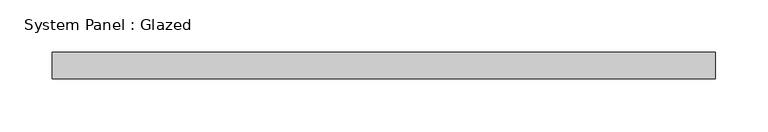
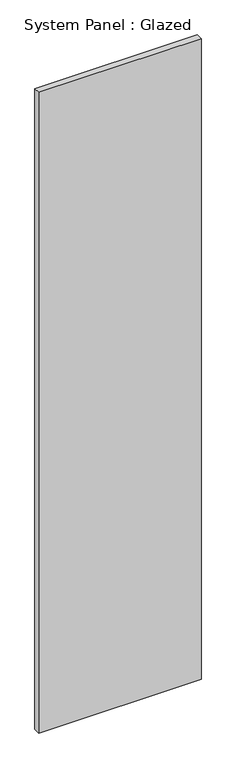
"""IFC4 building model written with IfcOpenShell, lengths in millimetres: plate geometry, System Panel : Glazed."""

from ifc_helpers import new_model, si_unit, origin, origin_with_axes, place, context, project, spatial, polyline, outline, extrude, source, transform, mapped, element, save


def system_panel_glazed_26227597(model_context):
    return source(origin(), model_context, "Body", "SweptSolid", [
        extrude(outline(polyline([(317.5, 19.05), (-317.5, 19.05), (-317.5, 44.45), (317.5, 44.45), (317.5, 19.05)])), origin_with_axes(), (0.0, 0.0, 1.0), 2647.95),
    ])


if __name__ == "__main__":
    model = new_model("IFC4")
    model_context = context("Model", 3, world=origin())
    ifc_project = project(units=[si_unit("LENGTHUNIT", "METRE", prefix="MILLI")], contexts=[model_context])
    site = spatial("IfcSite", under=ifc_project)
    building = spatial("IfcBuilding", under=site)
    placement = place(None, origin())
    system_panel_glazed_shape = system_panel_glazed_26227597(model_context)
    element("IfcPlate", 1, ObjectType="System Panel : Glazed", at=placement, inside=building, context=model_context, shape_type="MappedRepresentation", body=[
        mapped(system_panel_glazed_shape, transform((0.0, 0.0, 0.0), x_axis=(1.0, 0.0, 0.0), y_axis=(0.0, 1.0, 0.0), z_axis=(0.0, 0.0, 1.0))),
    ])
    save(model, "model.ifc")

# Revit data of these elements
# Type "System Panel : Glazed"
#   Construction Type Id = "GSP4R"
#   Analytic Construction = "1/8 in Pilkington single glazing"
#   Visual Light Transmittance = 0.9
#   Solar Heat Gain Coefficient = 0.86
#   Heat Transfer Coefficient (U) = 1.18115 BTU/(h·ft²·°F)
# Element 1 (IfcPlate, "System Panel : Glazed")
#   Materials on its faces: "Glass"
# Materials
#   "Glass": class "Glass", colour RGB 0 128 192, transparency 0.75, Description = "Soda Lime Glass", Cost = 0
